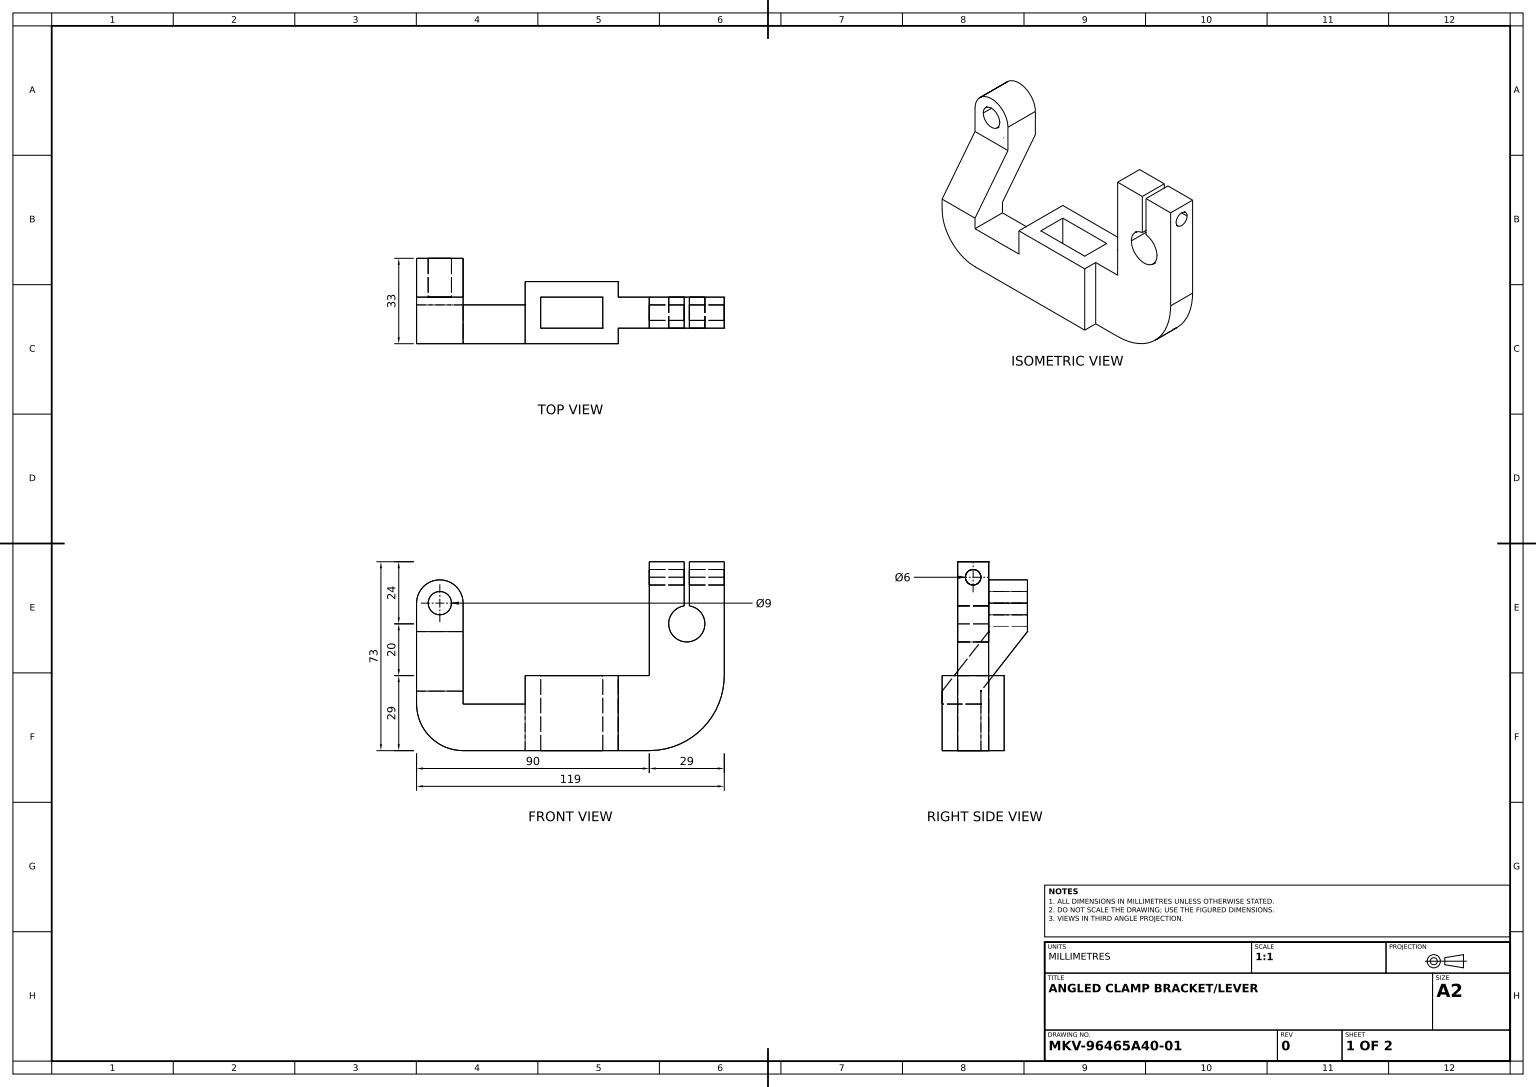
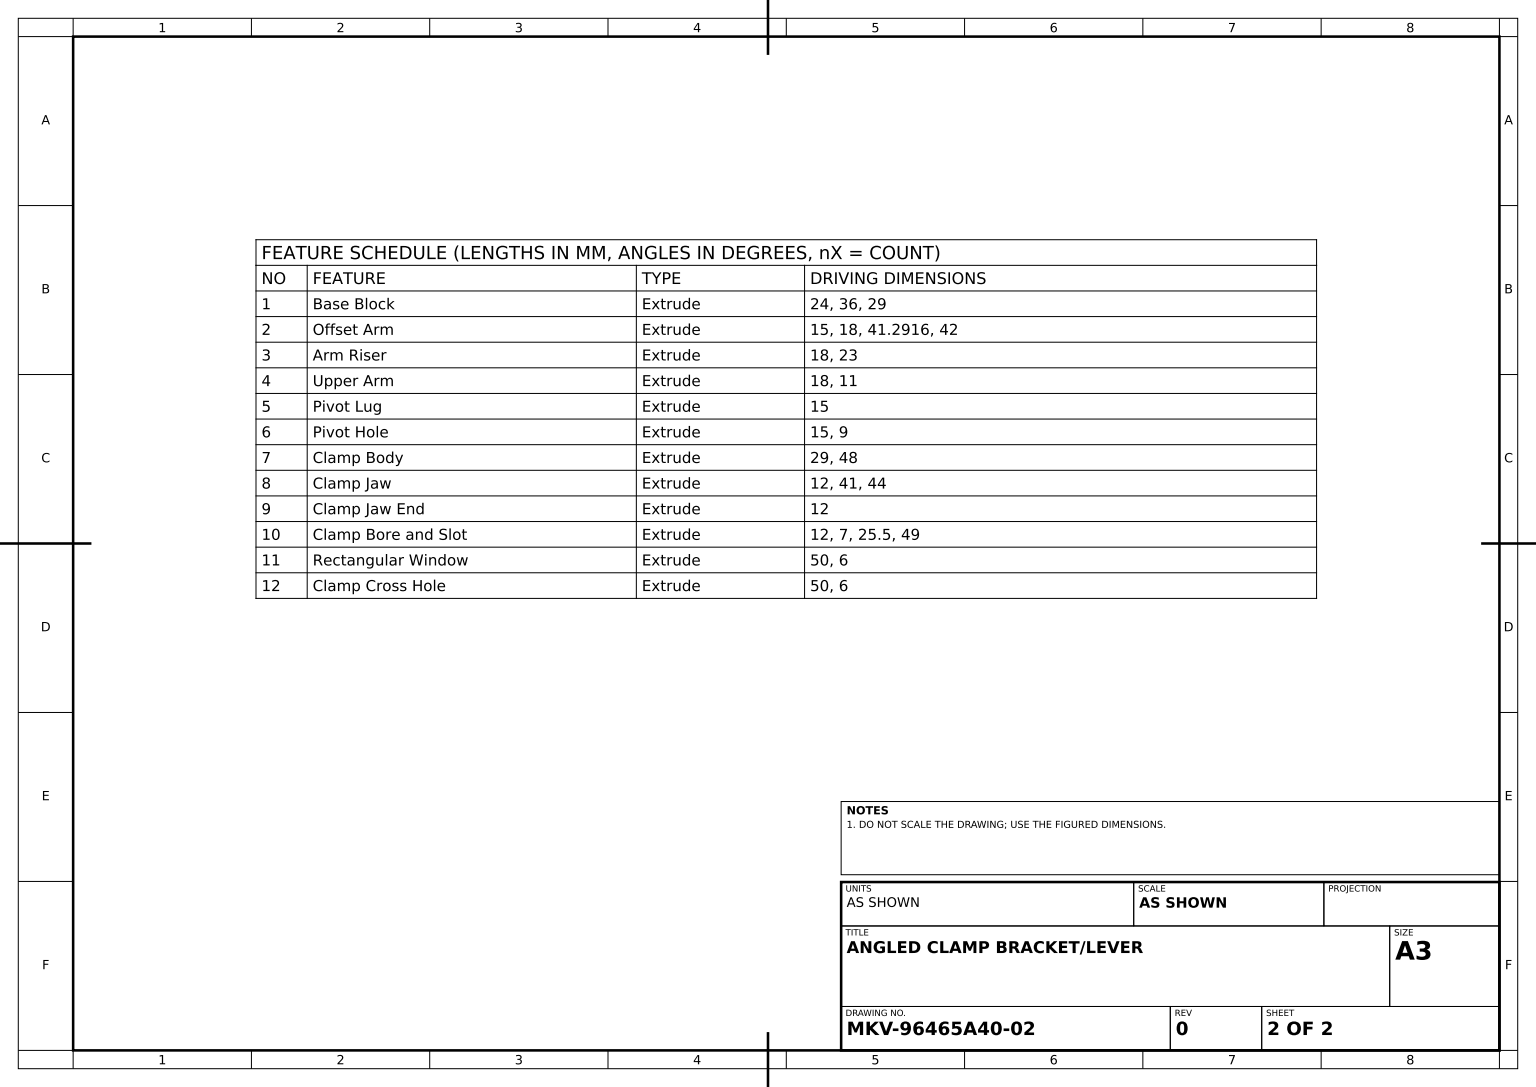
from build123d import *

# Parameters (mm, degrees)
BASE_BLOCK_SKETCH_W       = 36
BASE_BLOCK_SKETCH_H       = 29
BASE_BLOCK_DEPTH          = 24
OFFSET_ARM_DEPTH          = 15
ARM_RISER_DEPTH           = 18
UPPER_ARM_SKETCH_W        = 15
UPPER_ARM_SKETCH_H        = 11
UPPER_ARM_DEPTH           = 18
PIVOT_LUG_DEPTH           = 15
PIVOT_HOLE_SKETCH_R       = 4.5
PIVOT_HOLE_DEPTH          = 15
CLAMP_BODY_DEPTH          = 29
CLAMP_JAW_SKETCH_W        = 29
CLAMP_JAW_SKETCH_H        = 44
CLAMP_JAW_DEPTH           = 12
CLAMP_JAW_END_DEPTH       = 12
CLAMP_BORE_AND_SLOT_DEPTH = 12
WINDOW_SKETCH_W           = 24
WINDOW_SKETCH_H           = 12
RECTANGULAR_WINDOW_DEPTH  = 50
CROSS_HOLE_SKETCH_R       = 3
CLAMP_CROSS_HOLE_DEPTH    = 50


with BuildPart() as part:
    # Base Block Sketch → Base Block (new body)
    with BuildSketch(Plane.XY):
        with Locations((18, -14.5)):
            Rectangle(BASE_BLOCK_SKETCH_W, BASE_BLOCK_SKETCH_H)
    extrude(amount=BASE_BLOCK_DEPTH)

    # Offset Arm Sketch → Offset Arm (add)
    with BuildSketch(Plane.XY.offset(24)):
        with BuildLine():
            Line((0, -29), (-24, -29))
            ThreePointArc((-24, -29), (-36.727922061, -23.727922061), (-42, -11))
            Line((-42, -11), (-42, -6))
            Line((-42, -6), (-41.291616466, -6))
            Line((-41.291616466, -6), (-24, -6))
            Line((-24, -6), (-24, -11))
            Line((-24, -11), (0, -11))
            Line((0, -11), (0, -29))
        make_face()
    extrude(amount=-OFFSET_ARM_DEPTH)

    # Arm Riser Sketch → Arm Riser (add)
    with BuildSketch(Plane.ZY.offset(42)):
        Polygon((-9, 17), (9, -6), (24, -6), (6, 17), align=None)
    extrude(amount=-ARM_RISER_DEPTH)

    # Upper Arm Sketch → Upper Arm (add)
    with BuildSketch(Plane.ZY.offset(42)):
        with Locations((-1.5, 22.5)):
            Rectangle(UPPER_ARM_SKETCH_W, UPPER_ARM_SKETCH_H)
    extrude(amount=-UPPER_ARM_DEPTH)

    # Pivot Lug Sketch → Pivot Lug (add)
    with BuildSketch(Plane.XY.offset(6)):
        with BuildLine():
            Line((-42, 28), (-24, 28))
            ThreePointArc((-24, 28), (-33, 37), (-42, 28))
        make_face()
    extrude(amount=-PIVOT_LUG_DEPTH)

    # Pivot Hole Sketch → Pivot Hole (cut)
    with BuildSketch(Plane.XY.offset(6)):
        with Locations((-33, 28)):
            Circle(PIVOT_HOLE_SKETCH_R)
    extrude(amount=-PIVOT_HOLE_DEPTH, mode=Mode.SUBTRACT)

    # Clamp Body Sketch → Clamp Body (add)
    with BuildSketch(Plane(origin=(0, 0, 0), x_dir=(1, 0, 0), z_dir=(0, 1, 0))):
        Polygon((36, -6), (36, -12), (36, -18), (48, -18), (48, -6), align=None)
    extrude(amount=-CLAMP_BODY_DEPTH)



with BuildPart() as body_2:
    # Clamp Jaw Sketch → Clamp Jaw (new body)
    with BuildSketch(Plane.XY.offset(18)):
        with Locations((62.5, 22)):
            Rectangle(CLAMP_JAW_SKETCH_W, CLAMP_JAW_SKETCH_H)
    extrude(amount=-CLAMP_JAW_DEPTH)


with BuildPart() as part_1:
    add(part.part)

    add(body_2.part)  # Clamp Jaw End merges body 2
    # Clamp Jaw End Sketch → Clamp Jaw End (add)
    with BuildSketch(Plane.XY.offset(18)):
        with BuildLine():
            Line((48, 0), (77, 0))
            ThreePointArc((77, 0), (68.506096654, -20.506096654), (48, -29))
            Line((48, -29), (48, 0))
        make_face()
    extrude(amount=-CLAMP_JAW_END_DEPTH)

    # Clamp Bore Slot Sketch → Clamp Bore and Slot (cut)
    with BuildSketch(Plane.XY.offset(18)):
        with BuildLine():
            Line((62.5, 44), (61.5, 44))
            Line((61.5, 44), (61.5, 26.92820323))
            ThreePointArc((61.5, 26.92820323), (62.5, 13), (63.5, 26.92820323))
            Line((63.5, 26.92820323), (63.5, 44))
            Line((63.5, 44), (62.5, 44))
        make_face()
    extrude(amount=-CLAMP_BORE_AND_SLOT_DEPTH, mode=Mode.SUBTRACT)

    # Window Sketch → Rectangular Window (cut)
    with BuildSketch(Plane(origin=(0, 0, 0), x_dir=(1, 0, 0), z_dir=(0, 1, 0))):
        with Locations((18, -12)):
            Rectangle(WINDOW_SKETCH_W, WINDOW_SKETCH_H)
    extrude(amount=-RECTANGULAR_WINDOW_DEPTH, mode=Mode.SUBTRACT)

    # Cross Hole Sketch → Clamp Cross Hole (cut)
    with BuildSketch(Plane.ZY.offset(-48)):
        with Locations((12, 38)):
            Circle(CROSS_HOLE_SKETCH_R)
    extrude(amount=-CLAMP_CROSS_HOLE_DEPTH, mode=Mode.SUBTRACT)


solid = part_1.part
